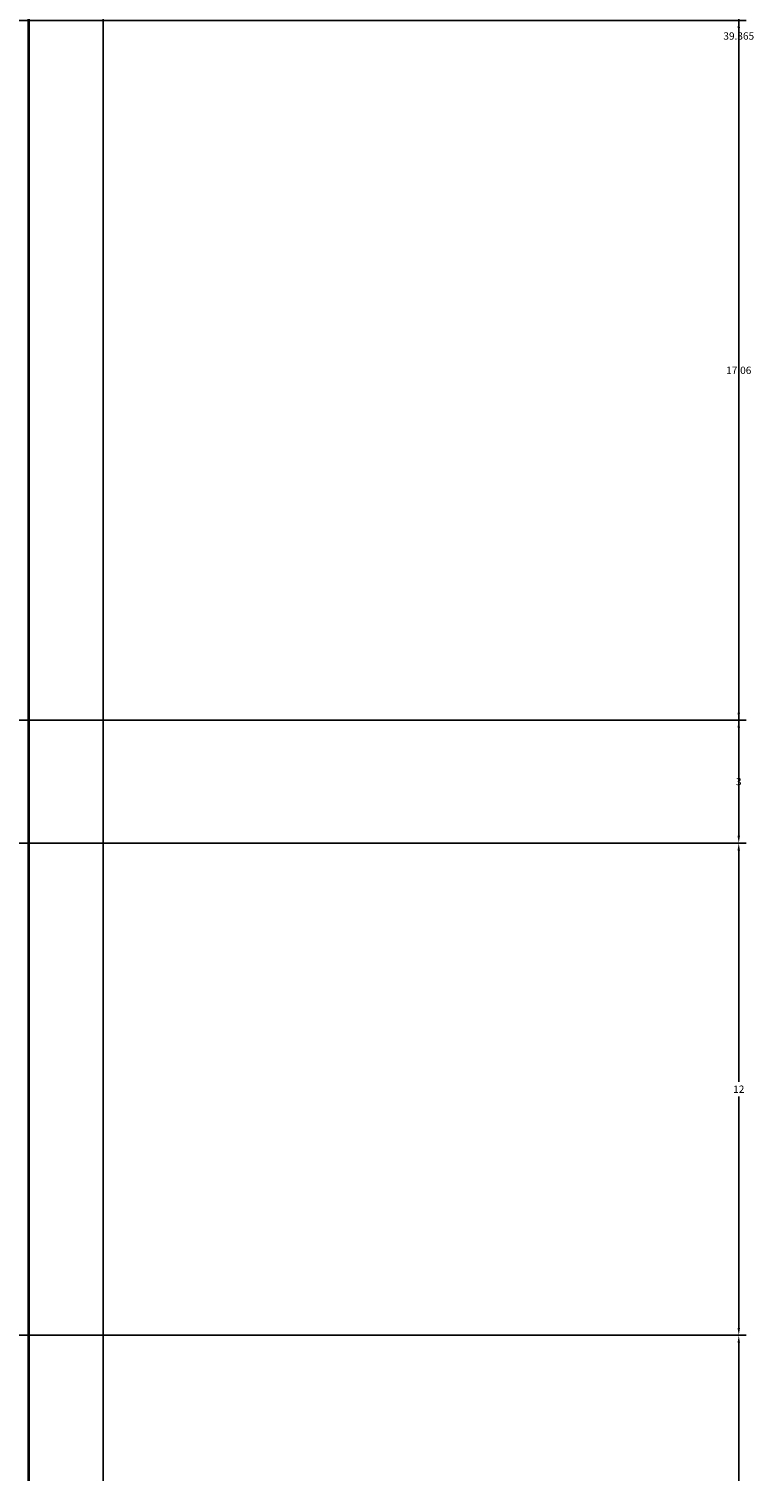
# Model space of a CAD drawing. Units: inches. Extents: x -6 to 289, y -8 to 323.
# Tile 66 of 107: x 271 to 289, y 124 to 159. Entities that reach past the tile are written whole.
import ezdxf

# ---------------------------------------------------------------- set-up
doc = ezdxf.new("R2010")
doc.units = ezdxf.units.IN
doc.header["$MEASUREMENT"] = 0
doc.layers.add('A-ANNO-DIMS', color=2, linetype='Continuous', lineweight=18)
doc.layers.add('A-ELEV', color=7, linetype='Continuous', lineweight=35)
doc.styles.get("Standard").update_dxf_attribs({"font": 'arial.ttf'})
doc.dimstyles.get("Standard").update_dxf_attribs({"dimtxt": 0.18, "dimasz": 0.18, "dimexe": 0.18, "dimexo": 0.0625, "dimgap": 0.09, "dimtad": 0, "dimtih": 1, "dimtoh": 1, "dimdec": 4, "dimzin": 0, "dimdsep": 46, "dimtxsty": 'Standard', "dimcen": 0.09, "dimadec": 0, "dimazin": 0, "dimtfac": 1, "dimtdec": 4, "dimtofl": 0, "dimtmove": 0, "dimatfit": 3, "dimfxl": 1, "dimtolj": 1, "dimtzin": 0, "dimarcsym": 0})

# ---------------------------------------------------------------- blocks, each defined once
blk = doc.blocks.new('*D23')
at = {"layer": 'A-ANNO-DIMS', "color": 0, "lineweight": -2, "transparency": 16777216}
for p, q in [((259.226, 127.289), (288.653, 127.289)), ((288.473, 127.109), (288.473, 67.471)), ((288.473, 7.469), (288.473, 67.107)), ((271.226, 7.289), (288.653, 7.289))]:
    blk.add_line(p, q, dxfattribs=at)
at = {"layer": 'A-ANNO-DIMS', "color": 0, "transparency": 16777216}
for points in [[(288.443, 127.109), (288.503, 127.109), (288.473, 127.289)], [(288.443, 7.469), (288.503, 7.469), (288.473, 7.289)]]:
    blk.add_solid(points, dxfattribs=at)
at = {"layer": 'Defpoints', "color": 0, "transparency": 16777216}
for p in [(259.164, 127.289), (288.473, 127.289), (271.164, 7.289)]:
    blk.add_point(p, dxfattribs=at)
at = {"layer": 'A-ANNO-DIMS', "color": 0, "transparency": 16777216, "insert": (288.473, 67.289), "char_height": 0.18, "attachment_point": 5}
blk.add_mtext('\\A1;120', dxfattribs=at)
blk = doc.blocks.new('*D24')
at = {"layer": 'A-ANNO-DIMS', "color": 0, "lineweight": -2, "transparency": 16777216}
for p, q in [((126.946, 178.654), (288.653, 178.654)), ((288.473, 178.474), (288.473, 159.153)), ((288.473, 139.469), (288.473, 158.789)), ((259.226, 139.289), (288.653, 139.289))]:
    blk.add_line(p, q, dxfattribs=at)
at = {"layer": 'A-ANNO-DIMS', "color": 0, "transparency": 16777216}
for points in [[(288.443, 178.474), (288.503, 178.474), (288.473, 178.654)], [(288.443, 139.469), (288.503, 139.469), (288.473, 139.289)]]:
    blk.add_solid(points, dxfattribs=at)
at = {"layer": 'Defpoints', "color": 0, "transparency": 16777216}
for p in [(126.883, 178.654), (288.473, 178.654), (259.164, 139.289)]:
    blk.add_point(p, dxfattribs=at)
at = {"layer": 'A-ANNO-DIMS', "color": 0, "transparency": 16777216, "insert": (288.473, 158.971), "char_height": 0.18, "attachment_point": 5}
blk.add_mtext('\\A1;39.365', dxfattribs=at)
blk = doc.blocks.new('*D82')
at = {"layer": 'A-ANNO-DIMS', "color": 0, "lineweight": -2, "transparency": 16777216}
for p, q in [((245.215, 66.286), (245.215, 322.969)), ((272.973, 66.286), (272.973, 322.969)), ((245.395, 322.789), (258.699, 322.789)), ((272.793, 322.789), (259.489, 322.789))]:
    blk.add_line(p, q, dxfattribs=at)
at = {"layer": 'A-ANNO-DIMS', "color": 0, "transparency": 16777216}
for points in [[(245.395, 322.819), (245.395, 322.759), (245.215, 322.789)], [(272.793, 322.819), (272.793, 322.759), (272.973, 322.789)]]:
    blk.add_solid(points, dxfattribs=at)
at = {"layer": 'Defpoints', "color": 0, "transparency": 16777216}
for p in [(272.973, 322.789), (245.215, 66.224), (272.973, 66.224)]:
    blk.add_point(p, dxfattribs=at)
at = {"layer": 'A-ANNO-DIMS', "color": 0, "transparency": 16777216, "insert": (259.094, 322.789), "char_height": 0.18, "attachment_point": 5}
blk.add_mtext('\\A1;27.76', dxfattribs=at)
blk = doc.blocks.new('*D101')
at = {"layer": 'A-ANNO-DIMS', "color": 0, "lineweight": -2, "transparency": 16777216}
for p, q in [((259.226, 139.289), (288.653, 139.289)), ((288.473, 139.109), (288.473, 133.469)), ((288.473, 127.469), (288.473, 133.108)), ((259.226, 127.289), (288.653, 127.289))]:
    blk.add_line(p, q, dxfattribs=at)
at = {"layer": 'A-ANNO-DIMS', "color": 0, "transparency": 16777216}
for points in [[(288.443, 139.109), (288.503, 139.109), (288.473, 139.289)], [(288.443, 127.469), (288.503, 127.469), (288.473, 127.289)]]:
    blk.add_solid(points, dxfattribs=at)
at = {"layer": 'Defpoints', "color": 0, "transparency": 16777216}
for p in [(259.164, 139.289), (288.473, 139.289), (259.164, 127.289)]:
    blk.add_point(p, dxfattribs=at)
at = {"layer": 'A-ANNO-DIMS', "color": 0, "transparency": 16777216, "insert": (288.473, 133.289), "char_height": 0.18, "attachment_point": 5}
blk.add_mtext('\\A1;12', dxfattribs=at)
blk = doc.blocks.new('*D102')
at = {"layer": 'A-ANNO-DIMS', "color": 0, "lineweight": -2, "transparency": 16777216}
for p, q in [((244.226, 142.289), (288.653, 142.289)), ((288.473, 142.109), (288.473, 140.971)), ((288.473, 139.469), (288.473, 140.607)), ((259.226, 139.289), (288.653, 139.289))]:
    blk.add_line(p, q, dxfattribs=at)
at = {"layer": 'A-ANNO-DIMS', "color": 0, "transparency": 16777216}
for points in [[(288.443, 142.109), (288.503, 142.109), (288.473, 142.289)], [(288.443, 139.469), (288.503, 139.469), (288.473, 139.289)]]:
    blk.add_solid(points, dxfattribs=at)
at = {"layer": 'Defpoints', "color": 0, "transparency": 16777216}
for p in [(244.164, 142.289), (288.473, 142.289), (259.164, 139.289)]:
    blk.add_point(p, dxfattribs=at)
at = {"layer": 'A-ANNO-DIMS', "color": 0, "transparency": 16777216, "insert": (288.473, 140.789), "char_height": 0.18, "attachment_point": 5}
blk.add_mtext('\\A1;3', dxfattribs=at)
blk = doc.blocks.new('*D103')
at = {"layer": 'A-ANNO-DIMS', "color": 0, "lineweight": -2, "transparency": 16777216}
for p, q in [((244.226, 159.348), (288.653, 159.348)), ((288.473, 159.168), (288.473, 151)), ((288.473, 142.469), (288.473, 150.637)), ((244.226, 142.289), (288.653, 142.289))]:
    blk.add_line(p, q, dxfattribs=at)
at = {"layer": 'A-ANNO-DIMS', "color": 0, "transparency": 16777216}
for points in [[(288.443, 159.168), (288.503, 159.168), (288.473, 159.348)], [(288.443, 142.469), (288.503, 142.469), (288.473, 142.289)]]:
    blk.add_solid(points, dxfattribs=at)
at = {"layer": 'Defpoints', "color": 0, "transparency": 16777216}
for p in [(244.164, 159.348), (288.473, 159.348), (244.164, 142.289)]:
    blk.add_point(p, dxfattribs=at)
at = {"layer": 'A-ANNO-DIMS', "color": 0, "transparency": 16777216, "insert": (288.473, 150.819), "char_height": 0.18, "attachment_point": 5}
blk.add_mtext('\\A1;17.06', dxfattribs=at)

msp = doc.modelspace()

# ---------------------------------------------------------------- linework, layer by layer
at = {"layer": 'A-ELEV'}
msp.add_line((271.1638, 68.4323), (271.1638, 259.2888), dxfattribs=at)

# ---------------------------------------------------------------- dimensions: what is measured, and where the dimension line sits
at = {"layer": 'A-ANNO-DIMS'}
dim = msp.add_linear_dim(base=(272.9733, 322.7888), p1=(245.2146, 66.2238), p2=(272.9733, 66.2238), dimstyle='Standard', override={"dimdec": 2, "dimlfac": 1, "dimrnd": 0, "dimzin": 0, "dimdsep": 46, "dimlunit": 2}, dxfattribs=at)
dim.commit()
dim.dimension.update_dxf_attribs({"geometry": '*D82', "text_midpoint": (259.0939, 322.7888)})
for base, p1, p2, override, picture, middle in [((288.4733, 178.654), (259.1638, 139.2888), (126.8835, 178.654), {"dimdec": 3, "dimlfac": 1, "dimrnd": 0, "dimzin": 0, "dimdsep": 46, "dimlunit": 2}, '*D24', (288.4733, 158.9714)), ((288.4733, 159.3484), (244.1638, 142.2888), (244.1638, 159.3484), {"dimdec": 2, "dimlfac": 1, "dimrnd": 0, "dimzin": 0, "dimdsep": 46, "dimlunit": 2}, '*D103', (288.4733, 150.8186)), ((288.4733, 142.2888), (259.1638, 139.2888), (244.1638, 142.2888), {"dimdec": 0, "dimlfac": 1, "dimrnd": 0, "dimzin": 0, "dimdsep": 46, "dimlunit": 2}, '*D102', (288.4733, 140.7888)), ((288.4733, 139.2888), (259.1638, 127.2888), (259.1638, 139.2888), {"dimdec": 0, "dimlfac": 1, "dimrnd": 0, "dimzin": 0, "dimdsep": 46, "dimlunit": 2}, '*D101', (288.4733, 133.2888)), ((288.4733, 127.2888), (271.1638, 7.2888), (259.1638, 127.2888), {"dimdec": 0, "dimlfac": 1, "dimrnd": 0, "dimzin": 0, "dimdsep": 46, "dimlunit": 2}, '*D23', (288.4733, 67.2888))]:
    dim = msp.add_linear_dim(base=base, p1=p1, p2=p2, angle=90, dimstyle='Standard', override=override, dxfattribs=at)
    dim.commit()
    dim.dimension.update_dxf_attribs({"geometry": picture, "text_midpoint": middle})

doc.saveas('drawing.dxf')
